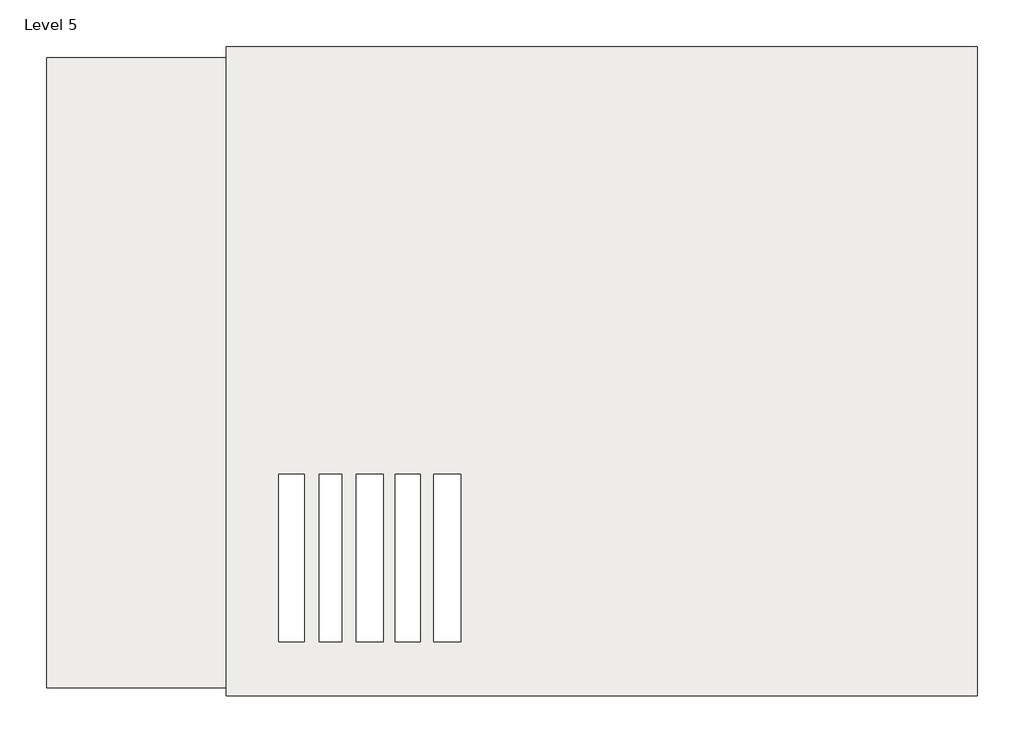
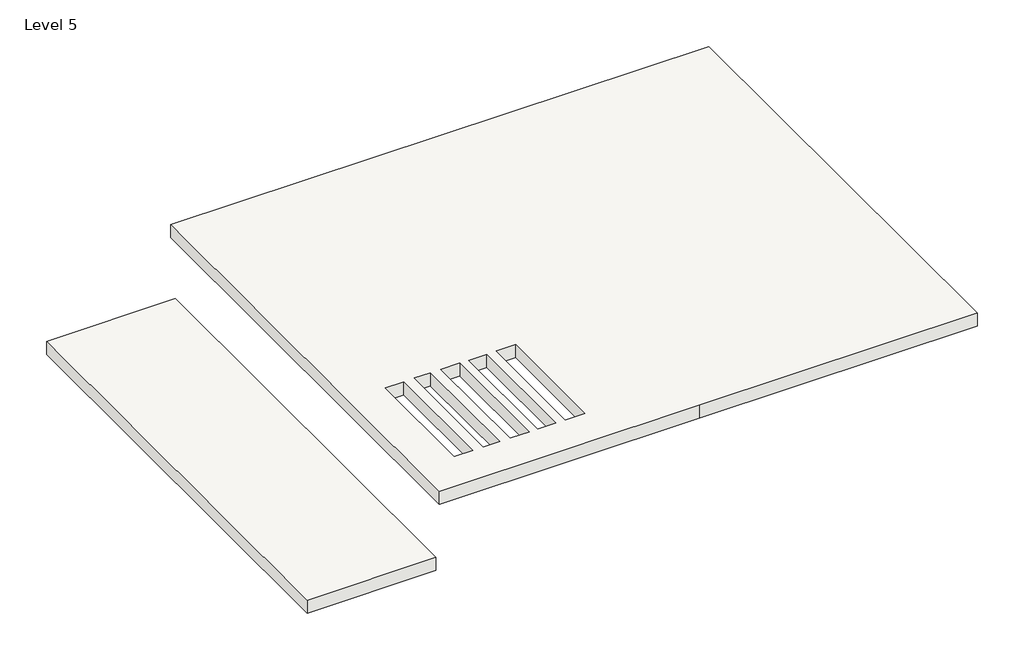
# One storey: 2 roofs.
"""IFC4 building model written with IfcOpenShell, lengths in millimetres."""

from ifc_helpers import new_model, si_unit, frame, origin, place, context, project, spatial, polyline, outline, extrude, element, save

model = new_model("IFC4")

# Units and contexts
model_context = context("Model", 3, world=origin())
ifc_project = project(units=[si_unit("LENGTHUNIT", "METRE", prefix="MILLI")], contexts=[model_context])

# Site, building, storey
site = spatial("IfcSite", under=ifc_project)
building = spatial("IfcBuilding", under=site)
storey = spatial("IfcBuildingStorey", under=building, Name="Level 5", Elevation=14630.4)

# Roofs
placement = place(None, origin())
element("IfcRoof", 1, ObjectType="Generic - 9\"", at=placement, inside=storey, context=model_context, shape_type="SweptSolid", body=[
    extrude(outline(polyline([(-14613.0593035, 12460.3935836), (-5710.3593035, 12460.3935836), (-5710.3593035, 4764.1935836), (-10301.4093035, 4764.1935836), (-14613.0593035, 4764.1935836), (-14613.0593035, 12460.3935836)]), holes=[polyline([(-13688.2094909, 5409.2962257), (-13688.2094909, 7390.4962257), (-13993.0094909, 7390.4962257), (-13993.0094909, 5409.2962257), (-13688.2094909, 5409.2962257)]), polyline([(-13243.6950294, 5409.2962257), (-13243.6950294, 7390.4962257), (-13511.8707314, 7390.4962257), (-13511.8707314, 5409.2962257), (-13243.6950294, 5409.2962257)]), polyline([(-12754.6687492, 5409.2962257), (-12754.6687492, 7390.4962257), (-13070.1695751, 7390.4962257), (-13070.1695751, 5409.2962257), (-12754.6687492, 5409.2962257)]), polyline([(-12312.9675929, 5409.2962257), (-12312.9675929, 7390.4962257), (-12612.6933775, 7390.4962257), (-12612.6933775, 5409.2962257), (-12312.9675929, 5409.2962257)]), polyline([(-11831.8288333, 5409.2962257), (-11831.8288333, 7390.4962257), (-12155.2171799, 7390.4962257), (-12155.2171799, 5409.2962257), (-11831.8288333, 5409.2962257)])]), frame((0.0, 0.0, 14630.4), z_axis=(0.0, 0.0, 1.0), x_axis=(1.0, 0.0, 0.0)), (0.0, 0.0, 1.0), 228.6),
])
element("IfcRoof", 2, ObjectType="Generic - 9\"", at=placement, inside=storey, context=model_context, shape_type="SweptSolid", body=[
    extrude(outline(polyline([(-16742.232922, 12329.8617654), (-14613.0593035, 12329.8617654), (-14613.0593035, 4862.2617654), (-16742.232922, 4862.2617654), (-16742.232922, 12329.8617654)])), frame((0.0, 0.0, 13411.2), z_axis=(0.0, 0.0, 1.0), x_axis=(1.0, 0.0, 0.0)), (0.0, 0.0, 1.0), 228.6),
])

save(model, "model.ifc")

# Revit data of these elements
# Type "Generic - 9\""
#   Assembly Code = "B1020"
#   Layers, outside or top first: 0' - 9" no material (function 1)
# Element 1 (IfcRoof, "Generic - 9\"")
#   built-in parameter 1001705 = 48.75 (stored number, unit not read)
#   built-in parameter 1001710 = 33615
#   Phase Created = New Construction
#   Materials on its faces: "Default Roof"
# Element 2 (IfcRoof, "Generic - 9\"")
#   built-in parameter 1001705 = 44.75 (stored number, unit not read)
#   built-in parameter 1001701 = -4 (stored number, unit not read)
#   built-in parameter 1001710 = 33615
#   Phase Created = New Construction
#   Materials on its faces: "Default Roof"
# Materials
#   "Default Roof": colour RGB 88 101 114, transparency 0
